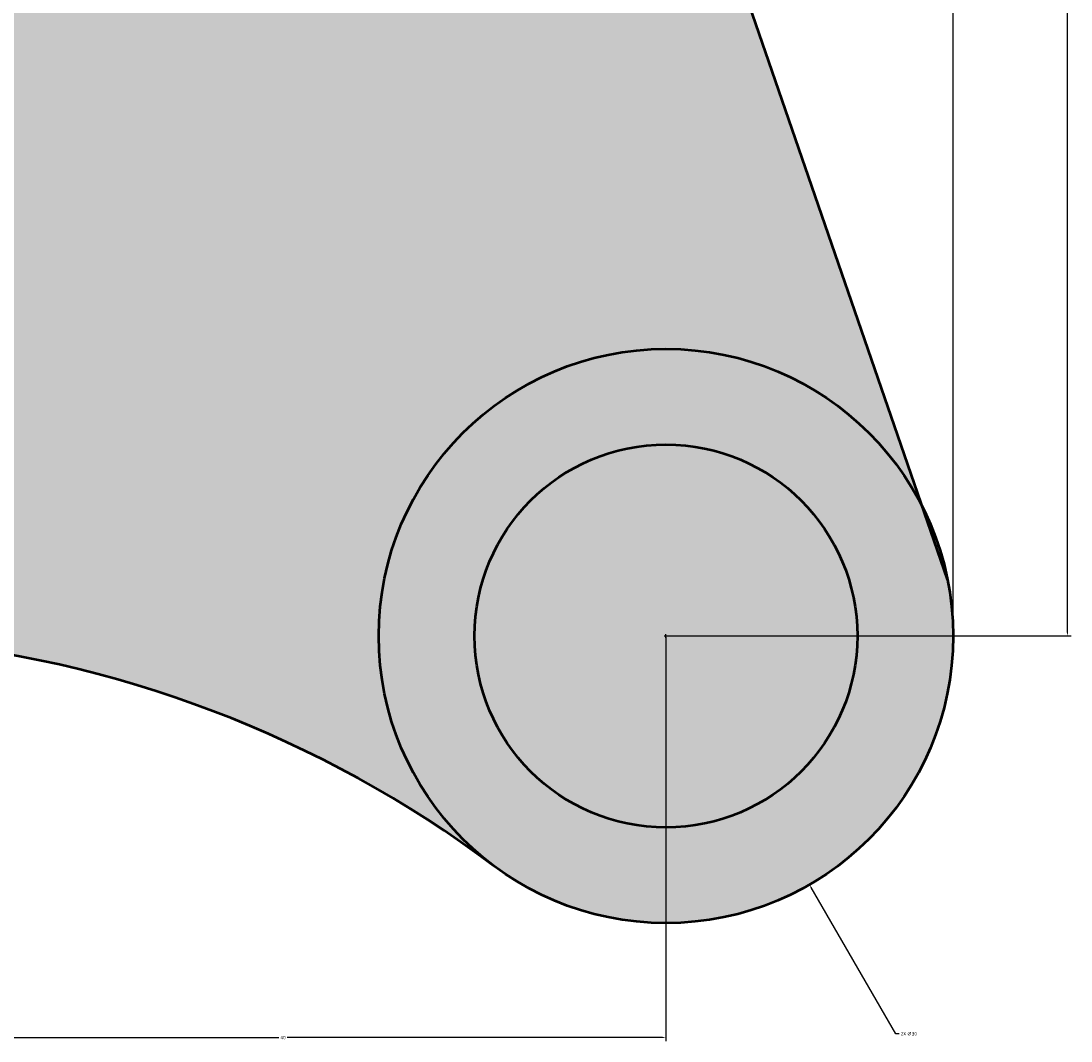
# Model space of a CAD drawing. Units: inches. Extents: x 114 to 236, y -51 to 115.
# Tile 4 of 14: x 182 to 236, y -12 to 41. Entities that reach past the tile are written whole.
import ezdxf

# ---------------------------------------------------------------- set-up
doc = ezdxf.new("R2010")
doc.units = ezdxf.units.IN
doc.header["$MEASUREMENT"] = 0
doc.layers.add('M-DIMS', color=2, linetype='Continuous', lineweight=18)
doc.layers.add('M-OUTL', color=7, linetype='Continuous', lineweight=50)
doc.layers.add('M-HATC', color=7, linetype='Continuous', lineweight=18, true_color=0xffffff)
doc.styles.get("Standard").update_dxf_attribs({"font": 'arial.ttf'})
doc.dimstyles.get("Standard").update_dxf_attribs({"dimtxt": 0.18, "dimasz": 0.18, "dimexe": 0.18, "dimexo": 0.0625, "dimgap": 0.09, "dimtad": 0, "dimtih": 1, "dimtoh": 1, "dimdec": 4, "dimzin": 0, "dimdsep": 46, "dimtxsty": 'Standard', "dimcen": 0.09, "dimadec": 0, "dimazin": 0, "dimtfac": 1, "dimtdec": 4, "dimtofl": 0, "dimtmove": 0, "dimatfit": 3, "dimfxl": 1, "dimtolj": 1, "dimtzin": 0, "dimarcsym": 0})

# ---------------------------------------------------------------- blocks, each defined once
blk = doc.blocks.new('BOSS-OD30-ID20')
for radius in [15, 10]:
    blk.add_circle((0, 0), radius)
blk = doc.blocks.new('*D3')
at = {"layer": 'Defpoints', "color": 0, "transparency": 16777216}
for p in [(230.229, 115.287), (120.229, 9.307), (230.229, 9.307)]:
    blk.add_point(p, dxfattribs=at)
at = {"layer": 'M-DIMS', "color": 0, "lineweight": -2, "transparency": 16777216}
for p, q in [((120.229, 9.37), (120.229, 115.467)), ((120.409, 115.287), (174.949, 115.287)), ((230.049, 115.287), (175.509, 115.287)), ((230.229, 9.37), (230.229, 115.467))]:
    blk.add_line(p, q, dxfattribs=at)
at = {"layer": 'M-DIMS', "color": 0, "transparency": 16777216}
for points in [[(120.409, 115.317), (120.409, 115.257), (120.229, 115.287)], [(230.049, 115.317), (230.049, 115.257), (230.229, 115.287)]]:
    blk.add_solid(points, dxfattribs=at)
at = {"layer": 'M-DIMS', "color": 0, "transparency": 16777216, "insert": (175.229, 115.287), "char_height": 0.18, "attachment_point": 5}
blk.add_mtext('\\A1;110', dxfattribs=at)
blk = doc.blocks.new('*D6')
at = {"layer": 'Defpoints', "color": 0, "transparency": 16777216}
for p in [(175.229, 79.307), (215.229, 9.307), (215.229, -11.673)]:
    blk.add_point(p, dxfattribs=at)
at = {"layer": 'M-DIMS', "color": 0, "lineweight": -2, "transparency": 16777216}
for p, q in [((175.229, 79.245), (175.229, -11.853)), ((215.229, 9.245), (215.229, -11.853)), ((175.409, -11.673), (195.006, -11.673)), ((215.049, -11.673), (195.451, -11.673))]:
    blk.add_line(p, q, dxfattribs=at)
at = {"layer": 'M-DIMS', "color": 0, "transparency": 16777216}
for points in [[(175.409, -11.643), (175.409, -11.703), (175.229, -11.673)], [(215.049, -11.643), (215.049, -11.703), (215.229, -11.673)]]:
    blk.add_solid(points, dxfattribs=at)
at = {"layer": 'M-DIMS', "color": 0, "transparency": 16777216, "insert": (195.229, -11.673), "char_height": 0.18, "attachment_point": 5}
blk.add_mtext('\\A1;40', dxfattribs=at)
blk = doc.blocks.new('*D7')
at = {"layer": 'Defpoints', "color": 0, "transparency": 16777216}
for p in [(175.229, 79.307), (236.209, 79.307), (215.229, 9.307)]:
    blk.add_point(p, dxfattribs=at)
at = {"layer": 'M-DIMS', "color": 0, "lineweight": -2, "transparency": 16777216}
for p, q in [((175.291, 79.307), (236.389, 79.307)), ((236.209, 79.127), (236.209, 44.489)), ((236.209, 9.487), (236.209, 44.125)), ((215.291, 9.307), (236.389, 9.307))]:
    blk.add_line(p, q, dxfattribs=at)
at = {"layer": 'M-DIMS', "color": 0, "transparency": 16777216}
for points in [[(236.179, 79.127), (236.239, 79.127), (236.209, 79.307)], [(236.179, 9.487), (236.239, 9.487), (236.209, 9.307)]]:
    blk.add_solid(points, dxfattribs=at)
at = {"layer": 'M-DIMS', "color": 0, "transparency": 16777216, "insert": (236.209, 44.307), "char_height": 0.18, "attachment_point": 5}
blk.add_mtext('\\A1;70', dxfattribs=at)
blk = doc.blocks.new('*D12')
at = {"layer": 'Defpoints', "color": 0, "transparency": 16777216}
for p in [(207.726, 22.296), (222.731, -3.682)]:
    blk.add_point(p, dxfattribs=at)
at = {"layer": 'M-DIMS', "color": 0, "lineweight": -2, "transparency": 16777216}
for p, q in [((215.229, 9.217), (215.229, 9.397)), ((215.139, 9.307), (215.319, 9.307)), ((227.233, -11.475), (222.821, -3.838)), ((227.413, -11.475), (227.233, -11.475))]:
    blk.add_line(p, q, dxfattribs=at)
at = {"layer": 'M-DIMS', "color": 0, "transparency": 16777216}
blk.add_solid([(222.847, -3.823), (222.795, -3.853), (222.731, -3.682)], dxfattribs=at)
at = {"layer": 'M-DIMS', "color": 0, "transparency": 16777216, "insert": (227.919, -11.475), "char_height": 0.18, "attachment_point": 5}
blk.add_mtext('\\A1;2X ∅30', dxfattribs=at)

msp = doc.modelspace()

# ---------------------------------------------------------------- hatches: boundary and pattern name
at = {"layer": 'M-HATC'}
h = msp.add_hatch(color=256, dxfattribs=at)
h.set_gradient(color1=(242, 103, 34), color2=(255, 255, 0), tint=1, name='INVSPHERICAL')
h.paths.add_polyline_path([(145.229, 79.307, -0.060651), (146.105, 86.505), (121.823, 16.038, -0.790743), (150.229, 9.307, -0.236068), (144.229, -2.693, -0.14094), (175.229, 9.098, -0.14094), (206.229, -2.693, -0.236068), (200.229, 9.307, -0.790743), (228.634, 16.038), (204.352, 86.505, -0.060651), (205.229, 79.307, -1)])
h = msp.add_hatch(color=256, dxfattribs=at)
h.set_gradient(color1=(19, 155, 72), color2=(255, 255, 0), tint=1, name='HEMISPHERICAL')
h.paths.add_polyline_path([(200.229, 9.307, 1), (230.229, 9.307, 0.049631), (229.935, 12.263), (228.634, 16.038, 0.790743)])
h.paths.add_polyline_path([(225.229, 9.307, -1), (205.229, 9.307, -1)], flags=16)
msp.add_hatch(color=256, dxfattribs=at).paths.add_polyline_path([(225.229, 9.307, 1), (205.229, 9.307, 1)])

# ---------------------------------------------------------------- linework, layer by layer
at = {"layer": 'M-OUTL'}
msp.add_line((229.935, 12.263), (202.605, 91.577), dxfattribs=at)
msp.add_arc((170.229, -50.693), 60, 53.1301, 85.21981, dxfattribs=at)

# ---------------------------------------------------------------- block references
msp.add_blockref('BOSS-OD30-ID20', (215.229, 9.307), dxfattribs=at)

# ---------------------------------------------------------------- dimensions: what is measured, and where the dimension line sits
at = {"layer": 'M-DIMS'}
for base, p1, p2, picture, middle in [((230.229, 115.287), (120.229, 9.307), (230.229, 9.307), '*D3', (175.229, 115.287)), ((215.229, -11.673), (175.229, 79.307), (215.229, 9.307), '*D6', (195.229, -11.673))]:
    dim = msp.add_linear_dim(base=base, p1=p1, p2=p2, dimstyle='Standard', override={"dimdec": 0, "dimlfac": 1, "dimrnd": 0, "dimzin": 0, "dimdsep": 46, "dimlunit": 2}, dxfattribs=at)
    dim.commit()
    dim.dimension.update_dxf_attribs({"geometry": picture, "text_midpoint": middle})
dim = msp.add_linear_dim(base=(236.209, 79.307), p1=(215.229, 9.307), p2=(175.229, 79.307), angle=90, dimstyle='Standard', override={"dimdec": 0, "dimlfac": 1, "dimrnd": 0, "dimzin": 0, "dimdsep": 46, "dimlunit": 2}, dxfattribs=at)
dim.commit()
dim.dimension.update_dxf_attribs({"geometry": '*D7', "text_midpoint": (236.209, 44.307)})
dim = msp.add_diameter_dim_2p(p1=(207.726, 22.296), p2=(222.731, -3.682), text='2X <>', dimstyle='Standard', override={"dimdec": 0, "dimlfac": 1, "dimrnd": 0, "dimzin": 0, "dimdsep": 46, "dimlunit": 2}, dxfattribs=at)
dim.commit()
dim.dimension.update_dxf_attribs({"geometry": '*D12', "text_midpoint": (227.919, -11.475), "dimtype": 163})

doc.saveas('drawing.dxf')
